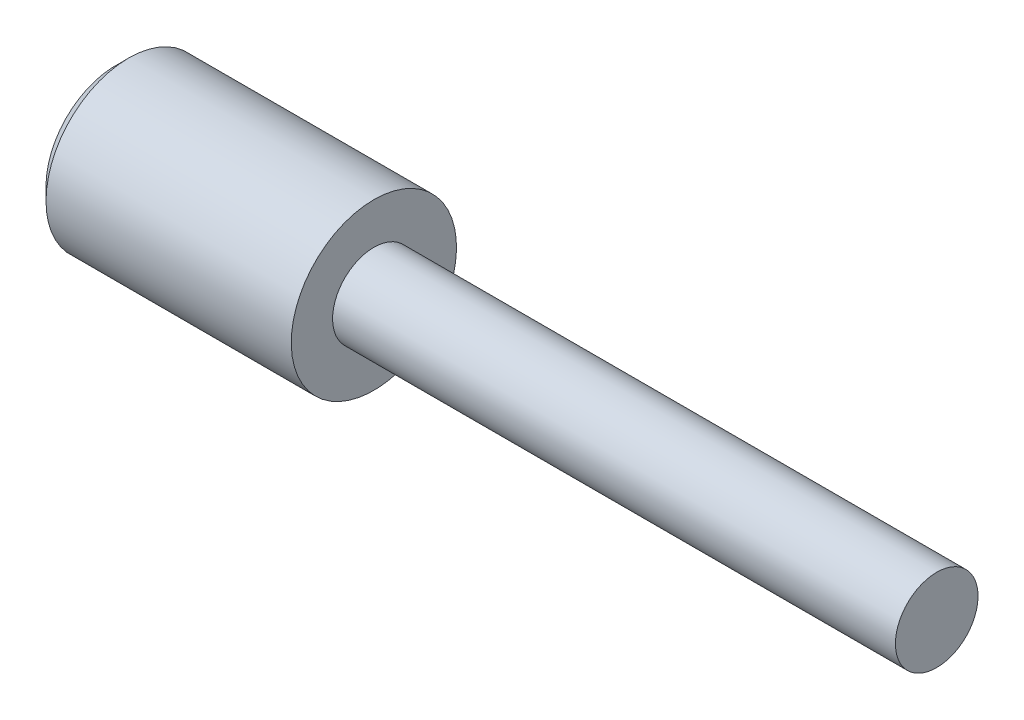
ISO-10303-21;
HEADER;
FILE_DESCRIPTION(('STEP AP214'),'2;1');
FILE_NAME('part.step','',(''),(''),'','','');
FILE_SCHEMA(('AUTOMOTIVE_DESIGN { 1 0 10303 214 1 1 1 1 }'));
ENDSEC;
DATA;
#1=APPLICATION_CONTEXT('core data for automotive mechanical design processes');
#2=APPLICATION_PROTOCOL_DEFINITION('international standard','automotive_design',2000,#1);
#3=PRODUCT_CONTEXT('',#1,'mechanical');
#4=PRODUCT('Part','Part','',(#3));
#5=PRODUCT_RELATED_PRODUCT_CATEGORY('part','',(#4));
#6=PRODUCT_DEFINITION_FORMATION('','',#4);
#7=PRODUCT_DEFINITION_CONTEXT('part definition',#1,'design');
#8=PRODUCT_DEFINITION('design','',#6,#7);
#9=PRODUCT_DEFINITION_SHAPE('','',#8);
#10=(LENGTH_UNIT() NAMED_UNIT(*) SI_UNIT(.MILLI.,.METRE.));
#11=(NAMED_UNIT(*) PLANE_ANGLE_UNIT() SI_UNIT($,.RADIAN.));
#12=(NAMED_UNIT(*) SI_UNIT($,.STERADIAN.) SOLID_ANGLE_UNIT());
#13=UNCERTAINTY_MEASURE_WITH_UNIT(LENGTH_MEASURE(1.E-05),#10,'distance_accuracy_value','');
#14=(GEOMETRIC_REPRESENTATION_CONTEXT(3) GLOBAL_UNCERTAINTY_ASSIGNED_CONTEXT((#13)) GLOBAL_UNIT_ASSIGNED_CONTEXT((#10,
#11,#12)) REPRESENTATION_CONTEXT('',''));
#15=CARTESIAN_POINT('',(0.,0.,0.));
#16=DIRECTION('',(0.,0.,1.));
#17=DIRECTION('',(1.,0.,0.));
#18=AXIS2_PLACEMENT_3D('',#15,#16,#17);
#19=CARTESIAN_POINT('',(-121.121212121212,34.3204688393368,0.));
#20=DIRECTION('',(1.,0.,0.));
#21=DIRECTION('',(0.,1.,0.));
#22=AXIS2_PLACEMENT_3D('',#19,#20,#21);
#23=PLANE('',#22);
#24=CARTESIAN_POINT('',(-121.121212121212,2.3204688393368,0.));
#25=DIRECTION('',(1.,0.,0.));
#26=DIRECTION('',(0.,1.,0.));
#27=AXIS2_PLACEMENT_3D('',#24,#25,#26);
#28=CIRCLE('',#27,32.);
#29=CARTESIAN_POINT('',(-121.121212121212,34.3204688393368,0.));
#30=VERTEX_POINT('',#29);
#31=EDGE_CURVE('E51',#30,#30,#28,.T.);
#32=ORIENTED_EDGE('',*,*,#31,.T.);
#33=EDGE_LOOP('',(#32));
#34=FACE_BOUND('',#33,.T.);
#35=CARTESIAN_POINT('',(-121.121212121212,2.3204688393368,0.));
#36=DIRECTION('',(1.,0.,0.));
#37=DIRECTION('',(0.,1.,0.));
#38=AXIS2_PLACEMENT_3D('',#35,#36,#37);
#39=CIRCLE('',#38,16.);
#40=CARTESIAN_POINT('',(-121.121212121212,18.3204688393368,0.));
#41=VERTEX_POINT('',#40);
#42=EDGE_CURVE('E58',#41,#41,#39,.T.);
#43=ORIENTED_EDGE('',*,*,#42,.F.);
#44=EDGE_LOOP('',(#43));
#45=FACE_BOUND('',#44,.T.);
#46=ADVANCED_FACE('F39',(#34,#45),#23,.T.);
#47=CARTESIAN_POINT('',(96.8787878787879,2.32046883933681,0.));
#48=DIRECTION('',(1.,0.,0.));
#49=DIRECTION('',(0.,1.,0.));
#50=AXIS2_PLACEMENT_3D('',#47,#48,#49);
#51=CYLINDRICAL_SURFACE('',#50,32.);
#52=CARTESIAN_POINT('',(-216.121212121212,2.32046883933679,0.));
#53=DIRECTION('',(-1.,0.,0.));
#54=DIRECTION('',(0.,-1.,0.));
#55=AXIS2_PLACEMENT_3D('',#52,#53,#54);
#56=CIRCLE('',#55,32.);
#57=CARTESIAN_POINT('',(-216.121212121212,-29.6795311606632,0.));
#58=VERTEX_POINT('',#57);
#59=EDGE_CURVE('E50',#58,#58,#56,.F.);
#60=ORIENTED_EDGE('',*,*,#59,.T.);
#61=EDGE_LOOP('',(#60));
#62=FACE_BOUND('',#61,.T.);
#63=ORIENTED_EDGE('',*,*,#31,.F.);
#64=EDGE_LOOP('',(#63));
#65=FACE_BOUND('',#64,.T.);
#66=ADVANCED_FACE('F70',(#62,#65),#51,.T.);
#67=CARTESIAN_POINT('',(-221.121212121212,34.3204688393368,0.));
#68=DIRECTION('',(-1.,0.,0.));
#69=DIRECTION('',(0.,-1.,0.));
#70=AXIS2_PLACEMENT_3D('',#67,#68,#69);
#71=PLANE('',#70);
#72=CARTESIAN_POINT('',(-221.121212121212,2.32046883933679,0.));
#73=DIRECTION('',(-1.,0.,0.));
#74=DIRECTION('',(0.,-1.,0.));
#75=AXIS2_PLACEMENT_3D('',#72,#73,#74);
#76=CIRCLE('',#75,26.9999999999999);
#77=CARTESIAN_POINT('',(-221.121212121212,-24.6795311606631,0.));
#78=VERTEX_POINT('',#77);
#79=EDGE_CURVE('E10',#78,#78,#76,.T.);
#80=ORIENTED_EDGE('',*,*,#79,.T.);
#81=EDGE_LOOP('',(#80));
#82=FACE_BOUND('',#81,.T.);
#83=ADVANCED_FACE('F74',(#82),#71,.T.);
#84=CARTESIAN_POINT('',(96.8787878787879,18.3204688393368,0.));
#85=DIRECTION('',(1.,0.,0.));
#86=DIRECTION('',(0.,1.,0.));
#87=AXIS2_PLACEMENT_3D('',#84,#85,#86);
#88=PLANE('',#87);
#89=CARTESIAN_POINT('',(96.8787878787879,2.32046883933681,0.));
#90=DIRECTION('',(1.,0.,0.));
#91=DIRECTION('',(0.,1.,0.));
#92=AXIS2_PLACEMENT_3D('',#89,#90,#91);
#93=CIRCLE('',#92,16.);
#94=CARTESIAN_POINT('',(96.8787878787879,18.3204688393368,0.));
#95=VERTEX_POINT('',#94);
#96=EDGE_CURVE('E54',#95,#95,#93,.T.);
#97=ORIENTED_EDGE('',*,*,#96,.T.);
#98=EDGE_LOOP('',(#97));
#99=FACE_BOUND('',#98,.T.);
#100=ADVANCED_FACE('F79',(#99),#88,.T.);
#101=CARTESIAN_POINT('',(96.8787878787879,2.32046883933681,0.));
#102=DIRECTION('',(1.,0.,0.));
#103=DIRECTION('',(0.,1.,0.));
#104=AXIS2_PLACEMENT_3D('',#101,#102,#103);
#105=CYLINDRICAL_SURFACE('',#104,16.);
#106=ORIENTED_EDGE('',*,*,#42,.T.);
#107=EDGE_LOOP('',(#106));
#108=FACE_BOUND('',#107,.T.);
#109=ORIENTED_EDGE('',*,*,#96,.F.);
#110=EDGE_LOOP('',(#109));
#111=FACE_BOUND('',#110,.T.);
#112=ADVANCED_FACE('F64',(#108,#111),#105,.T.);
#113=CARTESIAN_POINT('',(-216.121212121212,2.32046883933679,0.));
#114=DIRECTION('',(1.,0.,0.));
#115=DIRECTION('',(0.,1.,0.));
#116=AXIS2_PLACEMENT_3D('',#113,#114,#115);
#117=CONICAL_SURFACE('',#116,32.,0.785398163397452);
#118=ORIENTED_EDGE('',*,*,#79,.F.);
#119=EDGE_LOOP('',(#118));
#120=FACE_BOUND('',#119,.T.);
#121=ORIENTED_EDGE('',*,*,#59,.F.);
#122=EDGE_LOOP('',(#121));
#123=FACE_BOUND('',#122,.T.);
#124=ADVANCED_FACE('F45',(#120,#123),#117,.T.);
#125=CLOSED_SHELL('',(#46,#66,#83,#100,#112,#124));
#126=MANIFOLD_SOLID_BREP('B2',#125);
#127=ADVANCED_BREP_SHAPE_REPRESENTATION('',(#18,#126),#14);
#128=SHAPE_DEFINITION_REPRESENTATION(#9,#127);
ENDSEC;
END-ISO-10303-21;
